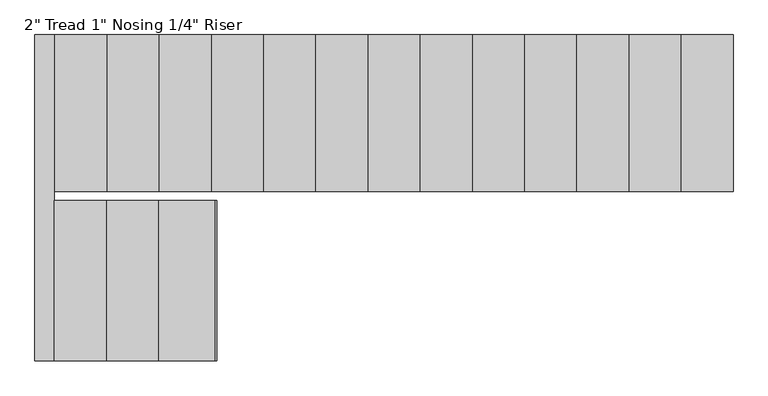
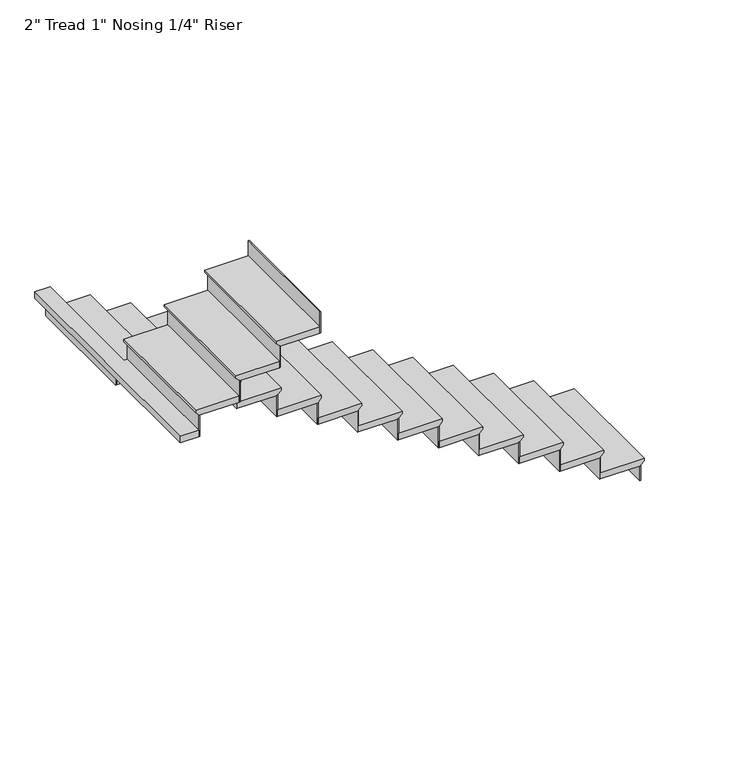
"""IFC4 building model written with IfcOpenShell, lengths in millimetres: stair flight geometry."""

from ifc_helpers import new_model, si_unit, origin, place, context, project, spatial, faceted_brep, source, transform, mapped, element, save


def stair_flight_3eca97f2(model_context):
    return source(origin(), model_context, "Body", "Brep", [
        faceted_brep([(6794.5, 11386.0372886, 9294.2833333), (6794.5, 11386.0372886, 9313.3333333), (6794.5, 10471.6372886, 9313.3333333), (6794.5, 10471.6372886, 9294.2833333), (6769.1, 11386.0372886, 9268.8833333), (6769.1, 10471.6372886, 9268.8833333), (6464.3, 11386.0372886, 9313.3333333), (6464.3, 10471.6372886, 9313.3333333), (6769.1, 10471.6372886, 9262.5333333), (6464.3, 10471.6372886, 9262.5333333), (6464.3, 11386.0372886, 9262.5333333), (6769.1, 11386.0372886, 9262.5333333)], [[[0, 1, 2, 3]], [[4, 0, 3, 5]], [[2, 1, 6, 7]], [[8, 9, 10, 11]], [[2, 7, 9, 8, 5, 3]], [[8, 11, 4, 5]], [[6, 1, 0, 4, 11, 10]], [[7, 6, 10, 9]]]),
        faceted_brep([(6769.1, 11386.0372886, 9262.5333333), (6769.1, 11386.0372886, 9144.0), (6762.75, 11386.0372886, 9144.0), (6762.75, 11386.0372886, 9262.5333333), (6769.1, 10471.6372886, 9262.5333333), (6762.75, 10471.6372886, 9262.5333333), (6762.75, 10471.6372886, 9144.0), (6769.1, 10471.6372886, 9144.0)], [[[0, 1, 2, 3]], [[4, 5, 6, 7]], [[1, 0, 4, 7]], [[2, 1, 7, 6]], [[3, 2, 6, 5]], [[0, 3, 5, 4]]]),
        faceted_brep([(6464.3, 11386.0372886, 9431.8666667), (6464.3, 11386.0372886, 9262.5333333), (6457.95, 11386.0372886, 9262.5333333), (6457.95, 11386.0372886, 9431.8666667), (6464.3, 10471.6372886, 9431.8666667), (6457.95, 10471.6372886, 9431.8666667), (6457.95, 10471.6372886, 9262.5333333), (6464.3, 10471.6372886, 9262.5333333)], [[[0, 1, 2, 3]], [[4, 5, 6, 7]], [[1, 0, 4, 7]], [[2, 1, 7, 6]], [[3, 2, 6, 5]], [[0, 3, 5, 4]]]),
        faceted_brep([(6489.7, 10471.6372886, 9482.6666667), (6489.7, 11386.0372886, 9482.6666667), (6159.5, 11386.0372886, 9482.6666667), (6159.5, 10471.6372886, 9482.6666667), (6464.3, 10471.6372886, 9431.8666667), (6159.5, 10471.6372886, 9431.8666667), (6159.5, 11386.0372886, 9431.8666667), (6464.3, 11386.0372886, 9431.8666667), (6464.3, 10471.6372886, 9438.2166667), (6489.7, 10471.6372886, 9463.6166667), (6464.3, 11386.0372886, 9438.2166667), (6489.7, 11386.0372886, 9463.6166667)], [[[0, 1, 2, 3]], [[4, 5, 6, 7]], [[0, 3, 5, 4, 8, 9]], [[4, 7, 10, 8]], [[2, 1, 11, 10, 7, 6]], [[3, 2, 6, 5]], [[11, 1, 0, 9]], [[10, 11, 9, 8]]]),
        faceted_brep([(6159.5, 11386.0372886, 9601.2), (6159.5, 11386.0372886, 9431.8666667), (6153.15, 11386.0372886, 9431.8666667), (6153.15, 11386.0372886, 9601.2), (6159.5, 10471.6372886, 9601.2), (6153.15, 10471.6372886, 9601.2), (6153.15, 10471.6372886, 9431.8666667), (6159.5, 10471.6372886, 9431.8666667)], [[[0, 1, 2, 3]], [[4, 5, 6, 7]], [[1, 0, 4, 7]], [[2, 1, 7, 6]], [[3, 2, 6, 5]], [[0, 3, 5, 4]]]),
        faceted_brep([(6184.9, 10471.6372886, 9652.0), (6184.9, 11386.0372886, 9652.0), (5854.7, 11386.0372886, 9652.0), (5854.7, 10471.6372886, 9652.0), (6159.5, 10471.6372886, 9601.2), (5854.7, 10471.6372886, 9601.2), (5854.7, 11386.0372886, 9601.2), (6159.5, 11386.0372886, 9601.2), (6159.5, 10471.6372886, 9607.55), (6184.9, 10471.6372886, 9632.95), (6159.5, 11386.0372886, 9607.55), (6184.9, 11386.0372886, 9632.95)], [[[0, 1, 2, 3]], [[4, 5, 6, 7]], [[0, 3, 5, 4, 8, 9]], [[4, 7, 10, 8]], [[2, 1, 11, 10, 7, 6]], [[3, 2, 6, 5]], [[11, 1, 0, 9]], [[10, 11, 9, 8]]]),
        faceted_brep([(5854.7, 11386.0372886, 9770.5333333), (5854.7, 11386.0372886, 9601.2), (5848.35, 11386.0372886, 9601.2), (5848.35, 11386.0372886, 9770.5333333), (5854.7, 10471.6372886, 9770.5333333), (5848.35, 10471.6372886, 9770.5333333), (5848.35, 10471.6372886, 9601.2), (5854.7, 10471.6372886, 9601.2)], [[[0, 1, 2, 3]], [[4, 5, 6, 7]], [[1, 0, 4, 7]], [[2, 1, 7, 6]], [[3, 2, 6, 5]], [[0, 3, 5, 4]]]),
        faceted_brep([(5880.1, 10471.6372886, 9821.3333333), (5880.1, 11386.0372886, 9821.3333333), (5549.9, 11386.0372886, 9821.3333333), (5549.9, 10471.6372886, 9821.3333333), (5854.7, 10471.6372886, 9770.5333333), (5549.9, 10471.6372886, 9770.5333333), (5549.9, 11386.0372886, 9770.5333333), (5854.7, 11386.0372886, 9770.5333333), (5854.7, 10471.6372886, 9776.8833333), (5880.1, 10471.6372886, 9802.2833333), (5854.7, 11386.0372886, 9776.8833333), (5880.1, 11386.0372886, 9802.2833333)], [[[0, 1, 2, 3]], [[4, 5, 6, 7]], [[0, 3, 5, 4, 8, 9]], [[4, 7, 10, 8]], [[2, 1, 11, 10, 7, 6]], [[3, 2, 6, 5]], [[11, 1, 0, 9]], [[10, 11, 9, 8]]]),
        faceted_brep([(5549.9, 11386.0372886, 9939.8666667), (5549.9, 11386.0372886, 9770.5333333), (5543.55, 11386.0372886, 9770.5333333), (5543.55, 11386.0372886, 9939.8666667), (5549.9, 10471.6372886, 9939.8666667), (5543.55, 10471.6372886, 9939.8666667), (5543.55, 10471.6372886, 9770.5333333), (5549.9, 10471.6372886, 9770.5333333)], [[[0, 1, 2, 3]], [[4, 5, 6, 7]], [[1, 0, 4, 7]], [[2, 1, 7, 6]], [[3, 2, 6, 5]], [[0, 3, 5, 4]]]),
        faceted_brep([(5575.3, 10471.6372886, 9990.6666667), (5575.3, 11386.0372886, 9990.6666667), (5245.1, 11386.0372886, 9990.6666667), (5245.1, 10471.6372886, 9990.6666667), (5549.9, 10471.6372886, 9939.8666667), (5245.1, 10471.6372886, 9939.8666667), (5245.1, 11386.0372886, 9939.8666667), (5549.9, 11386.0372886, 9939.8666667), (5549.9, 10471.6372886, 9946.2166667), (5575.3, 10471.6372886, 9971.6166667), (5549.9, 11386.0372886, 9946.2166667), (5575.3, 11386.0372886, 9971.6166667)], [[[0, 1, 2, 3]], [[4, 5, 6, 7]], [[0, 3, 5, 4, 8, 9]], [[4, 7, 10, 8]], [[2, 1, 11, 10, 7, 6]], [[3, 2, 6, 5]], [[11, 1, 0, 9]], [[10, 11, 9, 8]]]),
        faceted_brep([(5245.1, 11386.0372886, 10109.2), (5245.1, 11386.0372886, 9939.8666667), (5238.75, 11386.0372886, 9939.8666667), (5238.75, 11386.0372886, 10109.2), (5245.1, 10471.6372886, 10109.2), (5238.75, 10471.6372886, 10109.2), (5238.75, 10471.6372886, 9939.8666667), (5245.1, 10471.6372886, 9939.8666667)], [[[0, 1, 2, 3]], [[4, 5, 6, 7]], [[1, 0, 4, 7]], [[2, 1, 7, 6]], [[3, 2, 6, 5]], [[0, 3, 5, 4]]]),
        faceted_brep([(5270.5, 10471.6372886, 10160.0), (5270.5, 11386.0372886, 10160.0), (4940.3, 11386.0372886, 10160.0), (4940.3, 10471.6372886, 10160.0), (5245.1, 10471.6372886, 10109.2), (4940.3, 10471.6372886, 10109.2), (4940.3, 11386.0372886, 10109.2), (5245.1, 11386.0372886, 10109.2), (5245.1, 10471.6372886, 10115.55), (5270.5, 10471.6372886, 10140.95), (5245.1, 11386.0372886, 10115.55), (5270.5, 11386.0372886, 10140.95)], [[[0, 1, 2, 3]], [[4, 5, 6, 7]], [[0, 3, 5, 4, 8, 9]], [[4, 7, 10, 8]], [[2, 1, 11, 10, 7, 6]], [[3, 2, 6, 5]], [[11, 1, 0, 9]], [[10, 11, 9, 8]]]),
        faceted_brep([(4940.3, 11386.0372886, 10278.5333333), (4940.3, 11386.0372886, 10109.2), (4933.95, 11386.0372886, 10109.2), (4933.95, 11386.0372886, 10278.5333333), (4940.3, 10471.6372886, 10278.5333333), (4933.95, 10471.6372886, 10278.5333333), (4933.95, 10471.6372886, 10109.2), (4940.3, 10471.6372886, 10109.2)], [[[0, 1, 2, 3]], [[4, 5, 6, 7]], [[1, 0, 4, 7]], [[2, 1, 7, 6]], [[3, 2, 6, 5]], [[0, 3, 5, 4]]]),
        faceted_brep([(4965.7, 10471.6372886, 10329.3333333), (4965.7, 11386.0372886, 10329.3333333), (4635.5, 11386.0372886, 10329.3333333), (4635.5, 10471.6372886, 10329.3333333), (4940.3, 10471.6372886, 10278.5333333), (4635.5, 10471.6372886, 10278.5333333), (4635.5, 11386.0372886, 10278.5333333), (4940.3, 11386.0372886, 10278.5333333), (4940.3, 10471.6372886, 10284.8833333), (4965.7, 10471.6372886, 10310.2833333), (4940.3, 11386.0372886, 10284.8833333), (4965.7, 11386.0372886, 10310.2833333)], [[[0, 1, 2, 3]], [[4, 5, 6, 7]], [[0, 3, 5, 4, 8, 9]], [[4, 7, 10, 8]], [[2, 1, 11, 10, 7, 6]], [[3, 2, 6, 5]], [[11, 1, 0, 9]], [[10, 11, 9, 8]]]),
        faceted_brep([(4635.5, 11386.0372886, 10447.8666667), (4635.5, 11386.0372886, 10278.5333333), (4629.15, 11386.0372886, 10278.5333333), (4629.15, 11386.0372886, 10447.8666667), (4635.5, 10471.6372886, 10447.8666667), (4629.15, 10471.6372886, 10447.8666667), (4629.15, 10471.6372886, 10278.5333333), (4635.5, 10471.6372886, 10278.5333333)], [[[0, 1, 2, 3]], [[4, 5, 6, 7]], [[1, 0, 4, 7]], [[2, 1, 7, 6]], [[3, 2, 6, 5]], [[0, 3, 5, 4]]]),
        faceted_brep([(4660.9, 10471.6372886, 10498.6666667), (4660.9, 11386.0372886, 10498.6666667), (4330.7, 11386.0372886, 10498.6666667), (4330.7, 10471.6372886, 10498.6666667), (4635.5, 10471.6372886, 10447.8666667), (4330.7, 10471.6372886, 10447.8666667), (4330.7, 11386.0372886, 10447.8666667), (4635.5, 11386.0372886, 10447.8666667), (4635.5, 10471.6372886, 10454.2166667), (4660.9, 10471.6372886, 10479.6166667), (4635.5, 11386.0372886, 10454.2166667), (4660.9, 11386.0372886, 10479.6166667)], [[[0, 1, 2, 3]], [[4, 5, 6, 7]], [[0, 3, 5, 4, 8, 9]], [[4, 7, 10, 8]], [[2, 1, 11, 10, 7, 6]], [[3, 2, 6, 5]], [[11, 1, 0, 9]], [[10, 11, 9, 8]]]),
        faceted_brep([(4330.7, 11386.0372886, 10617.2), (4330.7, 11386.0372886, 10447.8666667), (4324.35, 11386.0372886, 10447.8666667), (4324.35, 11386.0372886, 10617.2), (4330.7, 10471.6372886, 10617.2), (4324.35, 10471.6372886, 10617.2), (4324.35, 10471.6372886, 10447.8666667), (4330.7, 10471.6372886, 10447.8666667)], [[[0, 1, 2, 3]], [[4, 5, 6, 7]], [[1, 0, 4, 7]], [[2, 1, 7, 6]], [[3, 2, 6, 5]], [[0, 3, 5, 4]]]),
        faceted_brep([(4356.1, 10471.6372886, 10668.0), (4356.1, 11386.0372886, 10668.0), (4025.9, 11386.0372886, 10668.0), (4025.9, 10471.6372886, 10668.0), (4330.7, 10471.6372886, 10617.2), (4025.9, 10471.6372886, 10617.2), (4025.9, 11386.0372886, 10617.2), (4330.7, 11386.0372886, 10617.2), (4330.7, 10471.6372886, 10623.55), (4356.1, 10471.6372886, 10648.95), (4330.7, 11386.0372886, 10623.55), (4356.1, 11386.0372886, 10648.95)], [[[0, 1, 2, 3]], [[4, 5, 6, 7]], [[0, 3, 5, 4, 8, 9]], [[4, 7, 10, 8]], [[2, 1, 11, 10, 7, 6]], [[3, 2, 6, 5]], [[11, 1, 0, 9]], [[10, 11, 9, 8]]]),
        faceted_brep([(4025.9, 11386.0372886, 10786.5333333), (4025.9, 11386.0372886, 10617.2), (4019.55, 11386.0372886, 10617.2), (4019.55, 11386.0372886, 10786.5333333), (4025.9, 10471.6372886, 10786.5333333), (4019.55, 10471.6372886, 10786.5333333), (4019.55, 10471.6372886, 10617.2), (4025.9, 10471.6372886, 10617.2)], [[[0, 1, 2, 3]], [[4, 5, 6, 7]], [[1, 0, 4, 7]], [[2, 1, 7, 6]], [[3, 2, 6, 5]], [[0, 3, 5, 4]]]),
        faceted_brep([(4051.3, 10471.6372886, 10837.3333333), (4051.3, 11386.0372886, 10837.3333333), (3721.1, 11386.0372886, 10837.3333333), (3721.1, 10471.6372886, 10837.3333333), (4025.9, 10471.6372886, 10786.5333333), (3721.1, 10471.6372886, 10786.5333333), (3721.1, 11386.0372886, 10786.5333333), (4025.9, 11386.0372886, 10786.5333333), (4025.9, 10471.6372886, 10792.8833333), (4051.3, 10471.6372886, 10818.2833333), (4025.9, 11386.0372886, 10792.8833333), (4051.3, 11386.0372886, 10818.2833333)], [[[0, 1, 2, 3]], [[4, 5, 6, 7]], [[0, 3, 5, 4, 8, 9]], [[4, 7, 10, 8]], [[2, 1, 11, 10, 7, 6]], [[3, 2, 6, 5]], [[11, 1, 0, 9]], [[10, 11, 9, 8]]]),
        faceted_brep([(3721.1, 11386.0372886, 10955.8666667), (3721.1, 11386.0372886, 10786.5333333), (3714.75, 11386.0372886, 10786.5333333), (3714.75, 11386.0372886, 10955.8666667), (3721.1, 10471.6372886, 10955.8666667), (3714.75, 10471.6372886, 10955.8666667), (3714.75, 10471.6372886, 10786.5333333), (3721.1, 10471.6372886, 10786.5333333)], [[[0, 1, 2, 3]], [[4, 5, 6, 7]], [[1, 0, 4, 7]], [[2, 1, 7, 6]], [[3, 2, 6, 5]], [[0, 3, 5, 4]]]),
        faceted_brep([(3746.5, 10471.6372886, 11006.6666667), (3746.5, 11386.0372886, 11006.6666667), (3416.3, 11386.0372886, 11006.6666667), (3416.3, 10471.6372886, 11006.6666667), (3721.1, 10471.6372886, 10955.8666667), (3416.3, 10471.6372886, 10955.8666667), (3416.3, 11386.0372886, 10955.8666667), (3721.1, 11386.0372886, 10955.8666667), (3721.1, 10471.6372886, 10962.2166667), (3746.5, 10471.6372886, 10987.6166667), (3721.1, 11386.0372886, 10962.2166667), (3746.5, 11386.0372886, 10987.6166667)], [[[0, 1, 2, 3]], [[4, 5, 6, 7]], [[0, 3, 5, 4, 8, 9]], [[4, 7, 10, 8]], [[2, 1, 11, 10, 7, 6]], [[3, 2, 6, 5]], [[11, 1, 0, 9]], [[10, 11, 9, 8]]]),
        faceted_brep([(3416.3, 11386.0372886, 11125.2), (3416.3, 11386.0372886, 10955.8666667), (3409.95, 11386.0372886, 10955.8666667), (3409.95, 11386.0372886, 11125.2), (3416.3, 10471.6372886, 11125.2), (3409.95, 10471.6372886, 11125.2), (3409.95, 10471.6372886, 10955.8666667), (3416.3, 10471.6372886, 10955.8666667)], [[[0, 1, 2, 3]], [[4, 5, 6, 7]], [[1, 0, 4, 7]], [[2, 1, 7, 6]], [[3, 2, 6, 5]], [[0, 3, 5, 4]]]),
        faceted_brep([(3441.7, 10471.6372886, 11176.0), (3441.7, 11386.0372886, 11176.0), (3111.5, 11386.0372886, 11176.0), (3111.5, 10471.6372886, 11176.0), (3416.3, 10471.6372886, 11125.2), (3111.5, 10471.6372886, 11125.2), (3111.5, 11386.0372886, 11125.2), (3416.3, 11386.0372886, 11125.2), (3416.3, 10471.6372886, 11131.55), (3441.7, 10471.6372886, 11156.95), (3416.3, 11386.0372886, 11131.55), (3441.7, 11386.0372886, 11156.95)], [[[0, 1, 2, 3]], [[4, 5, 6, 7]], [[0, 3, 5, 4, 8, 9]], [[4, 7, 10, 8]], [[2, 1, 11, 10, 7, 6]], [[3, 2, 6, 5]], [[11, 1, 0, 9]], [[10, 11, 9, 8]]]),
        faceted_brep([(3111.5, 11386.0372886, 11294.5333333), (3111.5, 11386.0372886, 11125.2), (3105.15, 11386.0372886, 11125.2), (3105.15, 11386.0372886, 11294.5333333), (3111.5, 10471.6372886, 11294.5333333), (3105.15, 10471.6372886, 11294.5333333), (3105.15, 10471.6372886, 11125.2), (3111.5, 10471.6372886, 11125.2)], [[[0, 1, 2, 3]], [[4, 5, 6, 7]], [[1, 0, 4, 7]], [[2, 1, 7, 6]], [[3, 2, 6, 5]], [[0, 3, 5, 4]]]),
        faceted_brep([(3136.9, 10471.6372886, 11345.3333333), (3136.9, 11386.0372886, 11345.3333333), (2806.7, 11386.0372886, 11345.3333333), (2806.7, 10471.6372886, 11345.3333333), (3111.5, 10471.6372886, 11294.5333333), (2806.7, 10471.6372886, 11294.5333333), (2806.7, 11386.0372886, 11294.5333333), (3111.5, 11386.0372886, 11294.5333333), (3111.5, 10471.6372886, 11300.8833333), (3136.9, 10471.6372886, 11326.2833333), (3111.5, 11386.0372886, 11300.8833333), (3136.9, 11386.0372886, 11326.2833333)], [[[0, 1, 2, 3]], [[4, 5, 6, 7]], [[0, 3, 5, 4, 8, 9]], [[4, 7, 10, 8]], [[2, 1, 11, 10, 7, 6]], [[3, 2, 6, 5]], [[11, 1, 0, 9]], [[10, 11, 9, 8]]]),
        faceted_brep([(2806.7, 11386.0372886, 11463.8666667), (2806.7, 11386.0372886, 11294.5333333), (2800.35, 11386.0372886, 11294.5333333), (2800.35, 11386.0372886, 11463.8666667), (2806.7, 10471.6372886, 11463.8666667), (2800.35, 10471.6372886, 11463.8666667), (2800.35, 10471.6372886, 11294.5333333), (2806.7, 10471.6372886, 11294.5333333)], [[[0, 1, 2, 3]], [[4, 5, 6, 7]], [[1, 0, 4, 7]], [[2, 1, 7, 6]], [[3, 2, 6, 5]], [[0, 3, 5, 4]]]),
        faceted_brep([(2857.5, 10418.2972886, 11514.6666667), (2832.1, 10418.2972886, 11514.6666667), (2832.1, 11386.0372886, 11514.6666667), (2717.8, 11386.0372886, 11514.6666667), (2717.8, 9481.0372886, 11514.6666667), (2857.5, 9481.0372886, 11514.6666667), (2832.1, 10418.2972886, 11463.8666667), (2857.5, 10418.2972886, 11463.8666667), (2857.5, 9481.0372886, 11463.8666667), (2717.8, 9481.0372886, 11463.8666667), (2717.8, 11386.0372886, 11463.8666667), (2806.7, 11386.0372886, 11463.8666667), (2806.7, 10471.6372886, 11463.8666667), (2832.1, 10471.6372886, 11463.8666667), (2832.1, 10471.6372886, 11495.6166667), (2832.1, 11386.0372886, 11495.6166667), (2806.7, 10471.6372886, 11470.2166667), (2806.7, 11386.0372886, 11470.2166667)], [[[0, 1, 2, 3, 4, 5]], [[6, 7, 8, 9, 10, 11, 12, 13]], [[1, 0, 7, 6]], [[2, 1, 6, 13, 14, 15]], [[13, 12, 16, 14]], [[12, 11, 17, 16]], [[3, 2, 15, 17, 11, 10]], [[4, 3, 10, 9]], [[5, 4, 9, 8]], [[0, 5, 8, 7]], [[17, 15, 14, 16]]]),
        faceted_brep([(2857.5, 9481.0372886, 11633.2), (2857.5, 9481.0372886, 11463.8666667), (2863.85, 9481.0372886, 11463.8666667), (2863.85, 9481.0372886, 11633.2), (2857.5, 10418.2972886, 11633.2), (2863.85, 10418.2972886, 11633.2), (2863.85, 10418.2972886, 11463.8666667), (2857.5, 10418.2972886, 11463.8666667)], [[[0, 1, 2, 3]], [[4, 5, 6, 7]], [[1, 0, 4, 7]], [[2, 1, 7, 6]], [[3, 2, 6, 5]], [[0, 3, 5, 4]]]),
        faceted_brep([(2832.1, 10418.2972886, 11684.0), (2832.1, 9481.0372886, 11684.0), (3162.3, 9481.0372886, 11684.0), (3162.3, 10418.2972886, 11684.0), (2857.5, 10418.2972886, 11633.2), (3162.3, 10418.2972886, 11633.2), (3162.3, 9481.0372886, 11633.2), (2857.5, 9481.0372886, 11633.2), (2857.5, 10418.2972886, 11639.55), (2832.1, 10418.2972886, 11664.95), (2857.5, 9481.0372886, 11639.55), (2832.1, 9481.0372886, 11664.95)], [[[0, 1, 2, 3]], [[4, 5, 6, 7]], [[0, 3, 5, 4, 8, 9]], [[4, 7, 10, 8]], [[2, 1, 11, 10, 7, 6]], [[3, 2, 6, 5]], [[11, 1, 0, 9]], [[10, 11, 9, 8]]]),
        faceted_brep([(3162.3, 9481.0372886, 11802.5333333), (3162.3, 9481.0372886, 11633.2), (3168.65, 9481.0372886, 11633.2), (3168.65, 9481.0372886, 11802.5333333), (3162.3, 10418.2972886, 11802.5333333), (3168.65, 10418.2972886, 11802.5333333), (3168.65, 10418.2972886, 11633.2), (3162.3, 10418.2972886, 11633.2)], [[[0, 1, 2, 3]], [[4, 5, 6, 7]], [[1, 0, 4, 7]], [[2, 1, 7, 6]], [[3, 2, 6, 5]], [[0, 3, 5, 4]]]),
        faceted_brep([(3136.9, 10418.2972886, 11853.3333333), (3136.9, 9481.0372886, 11853.3333333), (3467.1, 9481.0372886, 11853.3333333), (3467.1, 10418.2972886, 11853.3333333), (3162.3, 10418.2972886, 11802.5333333), (3467.1, 10418.2972886, 11802.5333333), (3467.1, 9481.0372886, 11802.5333333), (3162.3, 9481.0372886, 11802.5333333), (3162.3, 10418.2972886, 11808.8833333), (3136.9, 10418.2972886, 11834.2833333), (3162.3, 9481.0372886, 11808.8833333), (3136.9, 9481.0372886, 11834.2833333)], [[[0, 1, 2, 3]], [[4, 5, 6, 7]], [[0, 3, 5, 4, 8, 9]], [[4, 7, 10, 8]], [[2, 1, 11, 10, 7, 6]], [[3, 2, 6, 5]], [[11, 1, 0, 9]], [[10, 11, 9, 8]]]),
        faceted_brep([(3467.1, 9481.0372886, 11971.8666667), (3467.1, 9481.0372886, 11802.5333333), (3473.45, 9481.0372886, 11802.5333333), (3473.45, 9481.0372886, 11971.8666667), (3467.1, 10418.2972886, 11971.8666667), (3473.45, 10418.2972886, 11971.8666667), (3473.45, 10418.2972886, 11802.5333333), (3467.1, 10418.2972886, 11802.5333333)], [[[0, 1, 2, 3]], [[4, 5, 6, 7]], [[1, 0, 4, 7]], [[2, 1, 7, 6]], [[3, 2, 6, 5]], [[0, 3, 5, 4]]]),
        faceted_brep([(3771.9019847, 9481.0372886, 12141.2), (3771.9019847, 9481.0372886, 11971.8666667), (3778.2519847, 9481.0372886, 11971.8666667), (3778.2519847, 9481.0372886, 12141.2), (3771.9019847, 10418.2972886, 12141.2), (3778.2519847, 10418.2972886, 12141.2), (3778.2519847, 10418.2972886, 11971.8666667), (3771.9019847, 10418.2972886, 11971.8666667)], [[[0, 1, 2, 3]], [[4, 5, 6, 7]], [[1, 0, 4, 7]], [[2, 1, 7, 6]], [[3, 2, 6, 5]], [[0, 3, 5, 4]]]),
        faceted_brep([(3441.7, 10418.2972886, 12022.6666667), (3441.7, 9481.0372886, 12022.6666667), (3771.9019847, 9481.0372886, 12022.6666667), (3771.9019847, 10418.2972886, 12022.6666667), (3467.1, 10418.2972886, 11971.8666667), (3771.9019847, 10418.2972886, 11971.8666667), (3771.9019847, 9481.0372886, 11971.8666667), (3467.1, 9481.0372886, 11971.8666667), (3467.1, 10418.2972886, 11978.2166667), (3441.7, 10418.2972886, 12003.6166667), (3467.1, 9481.0372886, 11978.2166667), (3441.7, 9481.0372886, 12003.6166667)], [[[0, 1, 2, 3]], [[4, 5, 6, 7]], [[0, 3, 5, 4, 8, 9]], [[4, 7, 10, 8]], [[2, 1, 11, 10, 7, 6]], [[3, 2, 6, 5]], [[11, 1, 0, 9]], [[10, 11, 9, 8]]]),
    ])


if __name__ == "__main__":
    model = new_model("IFC4")
    model_context = context("Model", 3, world=origin())
    ifc_project = project(units=[si_unit("LENGTHUNIT", "METRE", prefix="MILLI")], contexts=[model_context])
    site = spatial("IfcSite", under=ifc_project)
    building = spatial("IfcBuilding", under=site)
    placement = place(None, origin())
    stair_flight_shape = stair_flight_3eca97f2(model_context)
    element("IfcStairFlight", 1, ObjectType="2\" Tread 1\" Nosing 1/4\" Riser", at=placement, inside=building, context=model_context, shape_type="MappedRepresentation", body=[
        mapped(stair_flight_shape, transform((0.0, 0.0, 0.0), x_axis=(1.0, 0.0, 0.0), y_axis=(0.0, 1.0, 0.0), z_axis=(0.0, 0.0, 1.0))),
    ])
    save(model, "model.ifc")
